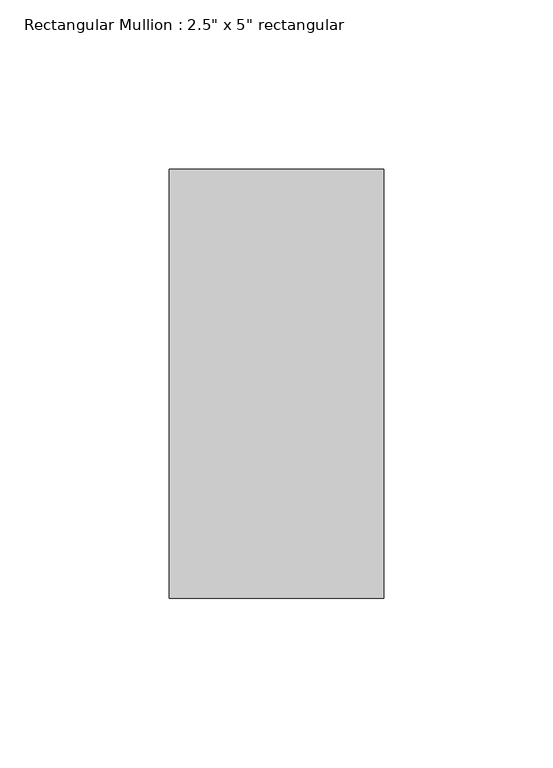
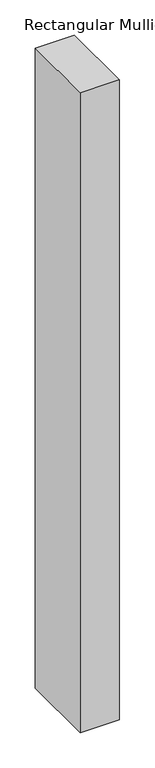
"""IFC4 building model written with IfcOpenShell, lengths in millimetres: member geometry."""

from ifc_helpers import new_model, si_unit, frame, origin, place, context, project, spatial, polyline, outline, extrude, source, transform, mapped, element, save


def member_3df3cfcf(model_context):
    return source(origin(), model_context, "Body", "SweptSolid", [
        extrude(outline(polyline([(31.75, 63.5), (31.75, -63.5), (-31.75, -63.5), (-31.75, 63.5), (31.75, 63.5)])), frame((0.0, 0.0, -1104.0913496), z_axis=(0.0, 0.0, 1.0), x_axis=(1.0, 0.0, 0.0)), (0.0, 0.0, 1.0), 1104.0913496),
    ])


if __name__ == "__main__":
    model = new_model("IFC4")
    model_context = context("Model", 3, world=origin())
    ifc_project = project(units=[si_unit("LENGTHUNIT", "METRE", prefix="MILLI")], contexts=[model_context])
    site = spatial("IfcSite", under=ifc_project)
    building = spatial("IfcBuilding", under=site)
    placement = place(None, origin())
    member_shape = member_3df3cfcf(model_context)
    element("IfcMember", 1, ObjectType="Rectangular Mullion : 2.5\" x 5\" rectangular", at=placement, inside=building, context=model_context, shape_type="MappedRepresentation", body=[
        mapped(member_shape, transform((0.0, 0.0, 0.0), x_axis=(1.0, 0.0, 0.0), y_axis=(0.0, 1.0, 0.0), z_axis=(0.0, 0.0, 1.0))),
    ])
    save(model, "model.ifc")

# Revit data of these elements
# Type "Rectangular Mullion : 2.5\" x 5\" rectangular"
#   built-in parameter 1007304 = 0.416667 (stored number, unit not read)
#   built-in parameter 1007301 = 0.104167 (stored number, unit not read)
#   built-in parameter 1007300 = 0.104167 (stored number, unit not read)
# Element 1 (IfcMember, "Rectangular Mullion : 2.5\" x 5\" rectangular")
#   Materials on its faces: "Aluminum"
# Materials
#   "Aluminum": class "Metal", colour RGB 247 247 247, transparency 0, Description = "Aluminum 6061", Cost = 0
